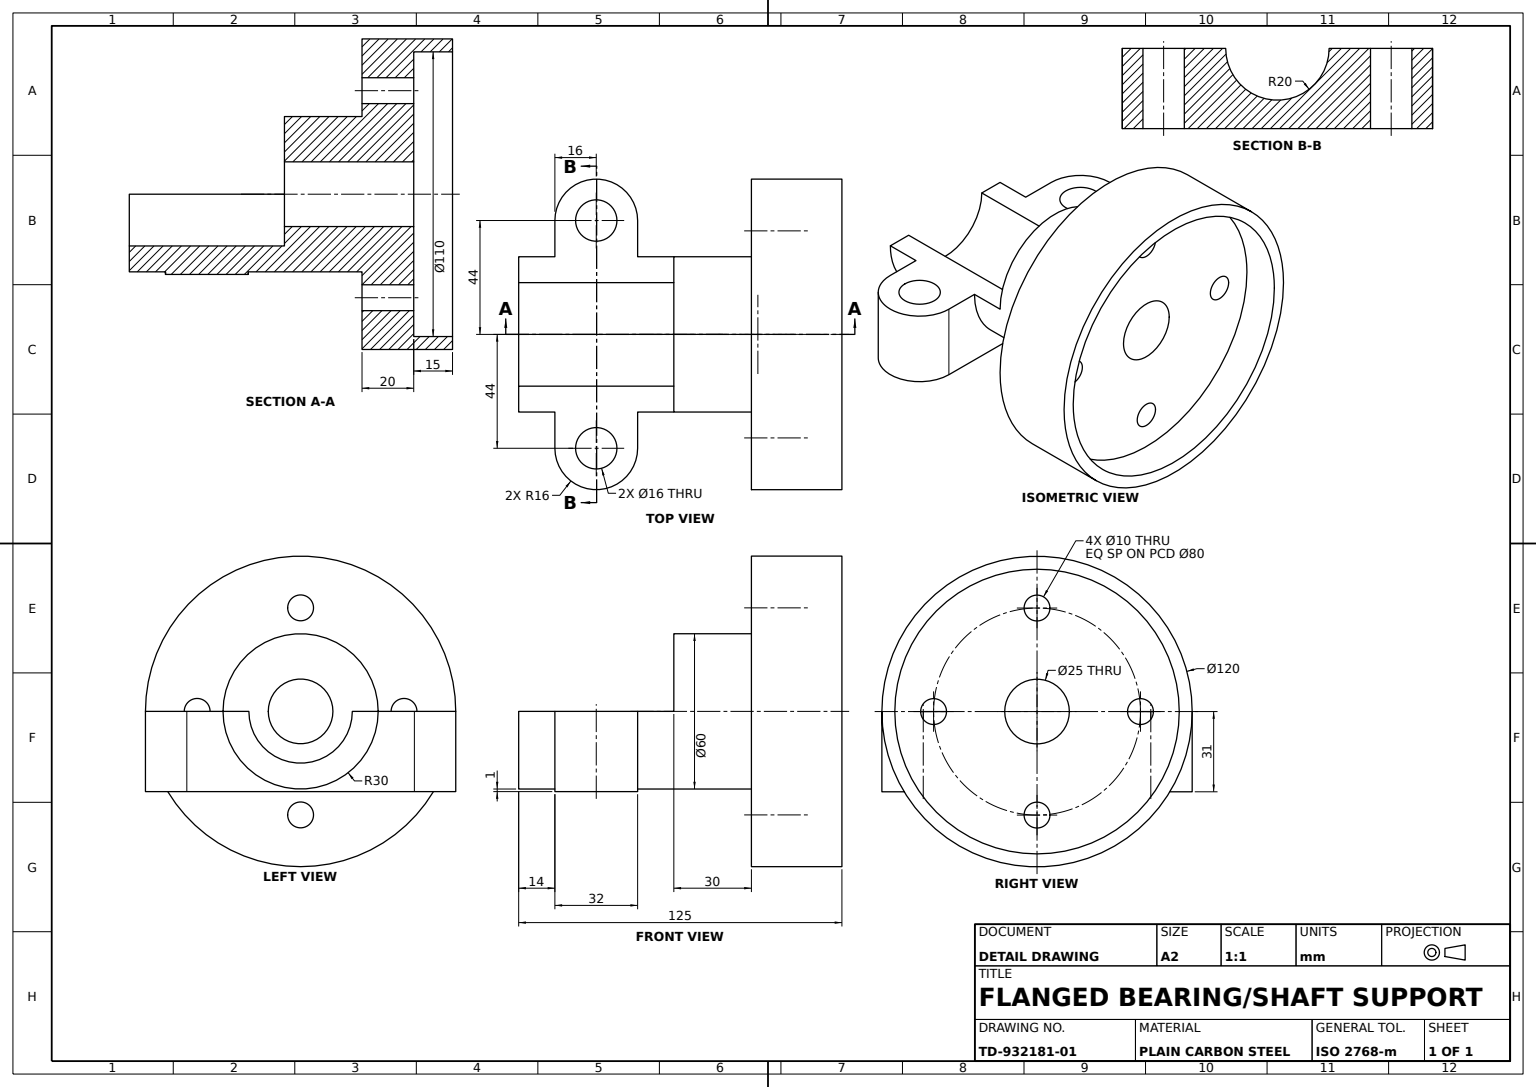
from build123d import *

# Parameters (mm, degrees)
BASE_FLANGE_SKETCH_R              = 60
BASE_FLANGE_SKETCH_R_2            = 55
BASE_FLANGE_PLATE_DEPTH           = 15
ROUND_FLANGE_SKETCH_120_R         = 60
ROUND_FLANGE_120_DEPTH            = 20
FLANGE_BOLT_HOLES_SKETCH_R        = 5
FLANGE_BOLT_HOLES_4X_10_DEPTH     = 20
HUB_BOSS_SKETCH_R                 = 30
HUB_BOSS_SKETCH_R_2               = 12.5
HUB_BOSS_DEPTH                    = 30
HUB_START                         = -30
HUB_BORE_SKETCH_25_R              = 12.5
HUB_BORE_25_DEPTH                 = 30
CRADLE_BODY_DEPTH                 = 60
CRADLE_LUGS_SKETCH_R              = 16
CRADLE_LUGS_SKETCH_R_2            = 8
CRADLE_MOUNTING_LUGS_DEPTH        = 31
CRADLE_BORE_SKETCH_40_R           = 20
CRADLE_BORE_40_DEPTH              = 60
LUG_PAD_SKETCH_R                  = 8
LUG_PADS_DEPTH                    = 32
PARTING_SLOT_SKETCH_W             = 120
PARTING_SLOT_SKETCH_H             = 1
CRADLE_PARTING_SLOT_1MM_DEPTH     = 32
LUG_BORE_SKETCH_40_R              = 20
CRADLE_BORE_40_THROUGH_LUGS_DEPTH = 60


with BuildPart() as part:
    # Base Flange Sketch → Base Flange Plate (new body)
    with BuildSketch(Plane.XY):
        Circle(BASE_FLANGE_SKETCH_R)
        Circle(BASE_FLANGE_SKETCH_R_2, mode=Mode.SUBTRACT)
    extrude(amount=BASE_FLANGE_PLATE_DEPTH)

    # Round Flange Sketch Ø120 → Round Flange Ø120 (add)
    with BuildSketch(Plane.XY.offset(15)):
        Circle(ROUND_FLANGE_SKETCH_120_R)
    extrude(amount=ROUND_FLANGE_120_DEPTH)

    # Flange Bolt Holes Sketch → Flange Bolt Holes 4xØ10 (cut)
    with BuildSketch(Plane.XY.offset(35)):
        with Locations((0, 40)):
            Circle(FLANGE_BOLT_HOLES_SKETCH_R)
        with Locations((40, 0)):
            Circle(FLANGE_BOLT_HOLES_SKETCH_R)
        with Locations((0, -40)):
            Circle(FLANGE_BOLT_HOLES_SKETCH_R)
        with Locations((-40, 0)):
            Circle(FLANGE_BOLT_HOLES_SKETCH_R)
    extrude(amount=-FLANGE_BOLT_HOLES_4X_10_DEPTH, mode=Mode.SUBTRACT)

    # Hub Boss Sketch → Hub Boss (add)
    with BuildSketch(Plane.XY.offset(35)):
        Circle(HUB_BOSS_SKETCH_R)
        Circle(HUB_BOSS_SKETCH_R_2, mode=Mode.SUBTRACT)
    extrude(amount=HUB_BOSS_DEPTH)

    # Hub Bore Sketch Ø25 → Hub Bore Ø25 (cut)
    with BuildSketch(Plane.XY.offset(35).offset(HUB_START)):
        Circle(HUB_BORE_SKETCH_25_R)
    extrude(amount=HUB_BORE_25_DEPTH, mode=Mode.SUBTRACT)

    # Cradle Body Sketch → Cradle Body (add)
    with BuildSketch(Plane.XY.offset(65)):
        with BuildLine():
            Line((-30, 0), (-12.5, 0))
            ThreePointArc((-12.5, 0), (0, -12.5), (12.5, 0))
            Line((12.5, 0), (30, 0))
            ThreePointArc((30, 0), (0, -30), (-30, 0))
        make_face()
    extrude(amount=CRADLE_BODY_DEPTH)


with BuildPart() as body_2:
    # Cradle Lugs Sketch → Cradle Mounting Lugs (new body)
    # profile 1 of 6: a face of its own
    with BuildSketch(Plane(origin=(0, 0, 0), x_dir=(1, 0, 0), z_dir=(0, 1, 0))):
        with Locations((-44, -95)):
            Circle(CRADLE_LUGS_SKETCH_R)
        with Locations(Location((-44, -95, 0), (0, 0, 270))):
            Circle(CRADLE_LUGS_SKETCH_R_2, mode=Mode.SUBTRACT)
    # profile 2 of 6: a face of its own
    with BuildSketch(Plane(origin=(0, 0, 0), x_dir=(1, 0, 0), z_dir=(0, 1, 0))):
        with BuildLine():
            Line((-12.5, -79), (-44, -79))
            ThreePointArc((-44, -79), (-32.686291501, -83.686291501), (-28, -95))
            ThreePointArc((-28, -95), (-32.686291501, -106.313708499), (-44, -111))
            Line((-44, -111), (-12.5, -111))
            Line((-12.5, -111), (12.5, -111))
            Line((12.5, -111), (12.5, -79))
            Line((12.5, -79), (-12.5, -79))
        make_face()
    # profile 3 of 6: a face of its own
    with BuildSketch(Plane(origin=(0, 0, 0), x_dir=(1, 0, 0), z_dir=(0, 1, 0))):
        with BuildLine():
            Line((30, -79), (12.5, -79))
            Line((12.5, -79), (12.5, -111))
            Line((12.5, -111), (30, -111))
            Line((30, -111), (30, -102.745966692))
            ThreePointArc((30, -102.745966692), (28, -95), (30, -87.254033308))
            Line((30, -87.254033308), (30, -79))
        make_face()
    # profile 4 of 6: a face of its own
    with BuildSketch(Plane(origin=(0, 0, 0), x_dir=(1, 0, 0), z_dir=(0, 1, 0))):
        with BuildLine():
            Line((44, -79), (30, -79))
            Line((30, -79), (30, -87.254033308))
            ThreePointArc((30, -87.254033308), (35.873975975, -81.217121725), (44, -79))
        make_face()
    # profile 5 of 6: a face of its own
    with BuildSketch(Plane(origin=(0, 0, 0), x_dir=(1, 0, 0), z_dir=(0, 1, 0))):
        with BuildLine():
            Line((30, -102.745966692), (30, -111))
            Line((30, -111), (44, -111))
            ThreePointArc((44, -111), (35.873975975, -108.782878275), (30, -102.745966692))
        make_face()
    # profile 6 of 6: a face of its own
    with BuildSketch(Plane(origin=(0, 0, 0), x_dir=(1, 0, 0), z_dir=(0, 1, 0))):
        with BuildLine():
            ThreePointArc((60, -95), (55.313708499, -83.686291501), (44, -79))
            ThreePointArc((44, -79), (35.873975975, -81.217121725), (30, -87.254033308))
            Line((30, -87.254033308), (30, -102.745966692))
            ThreePointArc((30, -102.745966692), (35.873975975, -108.782878275), (44, -111))
            ThreePointArc((44, -111), (55.313708499, -106.313708499), (60, -95))
        make_face()
        with Locations(Location((44, -95, 0), (0, 0, 270))):
            Circle(CRADLE_LUGS_SKETCH_R_2, mode=Mode.SUBTRACT)
    extrude(amount=-CRADLE_MOUNTING_LUGS_DEPTH)


with BuildPart() as cradle_bore_40_tool:
    # Cradle Bore Sketch Ø40 → Cradle Bore Ø40 (new body)
    with BuildSketch(Plane.XY.offset(125)):
        Circle(CRADLE_BORE_SKETCH_40_R)
    extrude(amount=-CRADLE_BORE_40_DEPTH)


with BuildPart() as part_1:
    add(part.part)

    # Cradle Bore Ø40: cut by cradle_bore_40_tool
    add(cradle_bore_40_tool.part, mode=Mode.SUBTRACT)



with BuildPart() as body_2_1:
    add(body_2.part)

    # Cradle Bore Ø40: cut by cradle_bore_40_tool
    add(cradle_bore_40_tool.part, mode=Mode.SUBTRACT)


with BuildPart() as part_2:
    add(part_1.part)

    add(body_2_1.part)  # Lug Pads merges body 2
    # Lug Pad Sketch → Lug Pads (add)
    # profile 1 of 4: a face of its own
    with BuildSketch(Plane.XZ.offset(31)):
        with BuildLine():
            ThreePointArc((-28, 95), (-32.686291501, 106.313708499), (-44, 111))
            ThreePointArc((-44, 111), (-60, 95), (-44, 79))
            ThreePointArc((-44, 79), (-32.686291501, 83.686291501), (-28, 95))
        make_face()
        with Locations(Location((-44, 95, 0), (0, 0, 270))):
            Circle(LUG_PAD_SKETCH_R, mode=Mode.SUBTRACT)
    # profile 2 of 4: a face of its own
    with BuildSketch(Plane.XZ.offset(31)):
        with BuildLine():
            Line((44, 111), (-44, 111))
            ThreePointArc((-44, 111), (-32.686291501, 106.313708499), (-28, 95))
            ThreePointArc((-28, 95), (-32.686291501, 83.686291501), (-44, 79))
            Line((-44, 79), (44, 79))
            ThreePointArc((44, 79), (35.873975975, 81.217121725), (30, 87.254033308))
            ThreePointArc((30, 87.254033308), (28, 95), (30, 102.745966692))
            ThreePointArc((30, 102.745966692), (35.873975975, 108.782878275), (44, 111))
        make_face()
    # profile 3 of 4: a face of its own
    with BuildSketch(Plane.XZ.offset(31)):
        with BuildLine():
            ThreePointArc((30, 87.254033308), (28, 95), (30, 102.745966692))
            Line((30, 102.745966692), (30, 87.254033308))
        make_face()
    # profile 4 of 4: a face of its own
    with BuildSketch(Plane.XZ.offset(31)):
        with BuildLine():
            ThreePointArc((60, 95), (55.313708499, 106.313708499), (44, 111))
            ThreePointArc((44, 111), (35.873975975, 108.782878275), (30, 102.745966692))
            Line((30, 102.745966692), (30, 87.254033308))
            ThreePointArc((30, 87.254033308), (35.873975975, 81.217121725), (44, 79))
            ThreePointArc((44, 79), (55.313708499, 83.686291501), (60, 95))
        make_face()
        with Locations(Location((44, 95, 0), (0, 0, 270))):
            Circle(LUG_PAD_SKETCH_R, mode=Mode.SUBTRACT)
    extrude(amount=-LUG_PADS_DEPTH)

    # Parting Slot Sketch → Cradle Parting Slot 1mm (cut)
    with BuildSketch(Plane.XY.offset(111)):
        with Locations((0, 0.5)):
            Rectangle(PARTING_SLOT_SKETCH_W, PARTING_SLOT_SKETCH_H)
    extrude(amount=-CRADLE_PARTING_SLOT_1MM_DEPTH, mode=Mode.SUBTRACT)

    # Lug Bore Sketch Ø40 → Cradle Bore Ø40 Through Lugs (cut)
    with BuildSketch(Plane.XY.offset(125)):
        Circle(LUG_BORE_SKETCH_40_R)
    extrude(amount=-CRADLE_BORE_40_THROUGH_LUGS_DEPTH, mode=Mode.SUBTRACT)


solid = part_2.part
